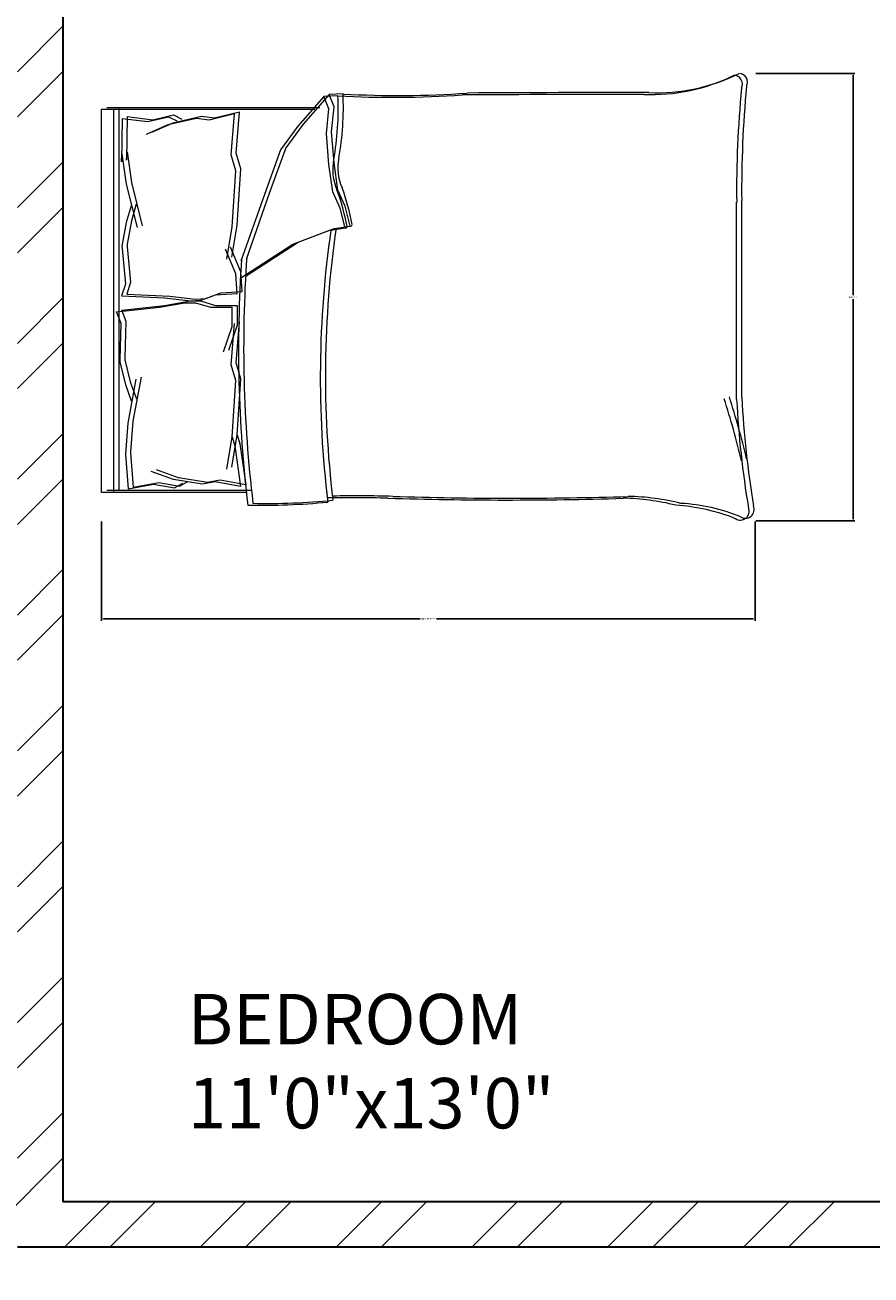
# Model space of a CAD drawing. Units: inches. Extents: x 1962 to 2771, y 1245 to 2660.
# Tile 107 of 114: x 2236 to 2319, y 2304 to 2428. Entities that reach past the tile are written whole.
import ezdxf

# ---------------------------------------------------------------- set-up
doc = ezdxf.new("R2010")
doc.units = ezdxf.units.IN
for name, color, linetype, lineweight in [('A-ANNO-DIMS', 2, 'Continuous', 18), ('A-AREA-IDEN', 7, 'Continuous', 18), ('A-FURN', 8, 'Continuous', 13), ('A-WALL', 7, 'Continuous', 35), ('A-WALL-PATT', 252, 'Continuous', 13)]:
    doc.layers.add(name, color=color, linetype=linetype, lineweight=lineweight)
doc.styles.get("Standard").update_dxf_attribs({"font": 'arial.ttf'})
doc.dimstyles.get("Standard").update_dxf_attribs({"dimtxt": 0.18, "dimasz": 0.18, "dimexe": 0.18, "dimexo": 0.0625, "dimgap": 0.09, "dimtad": 0, "dimtih": 1, "dimtoh": 1, "dimdec": 4, "dimzin": 0, "dimdsep": 46, "dimtxsty": 'Standard', "dimcen": 0.09, "dimadec": 0, "dimazin": 0, "dimtfac": 1, "dimtdec": 4, "dimtofl": 0, "dimtmove": 0, "dimatfit": 3, "dimfxl": 1, "dimtolj": 1, "dimtzin": 0, "dimarcsym": 0})

# ---------------------------------------------------------------- blocks, each defined once
blk = doc.blocks.new('BED-PLAN')
for p, q in [((22.56, 42.21), (19.98, 39.26)), ((22.56, 42.21), (19.98, 39.26)), ((23.95, 42.27), (22.56, 42.21, 3.08)), ((23.95, 42.27), (22.56, 42.21, 3.08)), ((23.06, 40.98), (22.56, 42.21)), ((23.06, 40.98), (22.56, 42.21)), ((0.51, 40.93), (21.66, 40.93)), ((0.51, 40.93), (21.66, 40.93)), ((1.73, 2.95), (1.73, 40.93)), ((1.73, 2.95), (1.73, 40.93)), ((22.05, 42.03), (19.47, 39.08)), ((22.05, 42.02), (19.47, 39.08)), ((23.44, 42.09), (22.05, 42.03, 3.08)), ((23.44, 42.09), (22.05, 42.02, 3.08)), ((22.55, 40.8), (22.05, 42.03)), ((22.55, 40.8), (22.05, 42.02)), ((22.81, 38.52), (23.06, 40.98)), ((22.81, 38.52), (23.06, 40.98)), ((0, 40.75), (21.15, 40.75)), ((0, 40.75), (21.15, 40.75)), ((0, 2.76), (0, 40.75)), ((1.22, 2.76), (1.22, 40.75)), ((1.22, 2.76), (1.22, 40.75)), ((2.03, 39.83), (1.96, 35.54)), ((2.03, 39.83), (1.96, 35.54)), ((2.03, 39.83), (4.58, 39.53)), ((2.03, 39.83), (4.58, 39.53)), ((2.54, 40.02), (2.46, 35.72)), ((2.54, 40.02), (2.46, 35.72)), ((2.54, 40.02), (5.09, 39.72)), ((2.54, 40.02), (5.09, 39.72)), ((4.58, 39.53), (6.63, 40.01)), ((4.58, 39.53), (6.63, 40.01)), ((5.09, 39.72), (7.14, 40.19)), ((5.09, 39.72), (7.14, 40.19)), ((9.4, 39.83), (6.56, 39.2)), ((9.4, 39.83), (6.56, 39.2)), ((6.63, 40.01), (7.46, 39.6)), ((6.63, 40.01), (7.46, 39.6)), ((9.91, 40.02), (7.07, 39.38)), ((9.91, 40.02), (7.07, 39.38)), ((7.14, 40.19), (7.97, 39.78)), ((7.14, 40.19), (7.97, 39.78)), ((10.68, 39.68), (9.4, 39.83)), ((10.68, 39.68), (9.4, 39.83)), ((11.19, 39.87), (9.91, 40.02)), ((11.19, 39.87), (9.91, 40.02)), ((13.17, 40.3), (10.68, 39.68)), ((13.17, 40.3), (10.68, 39.68)), ((13.68, 40.48), (11.19, 39.87)), ((13.68, 40.48), (11.19, 39.87)), ((12.85, 36.22), (13.17, 40.3)), ((12.85, 36.22), (13.17, 40.3)), ((13.36, 36.4), (13.68, 40.48)), ((13.36, 36.4), (13.68, 40.48)), ((22.3, 38.34), (22.55, 40.8)), ((22.3, 38.34), (22.55, 40.8)), ((6.56, 39.2), (4.43, 38.26)), ((6.56, 39.2), (4.43, 38.26)), ((7.07, 39.38), (4.94, 38.44)), ((7.07, 39.38), (4.94, 38.44)), ((19.47, 39.08), (17.75, 36.74)), ((19.47, 39.08), (17.75, 36.74)), ((19.98, 39.26), (18.26, 36.92)), ((19.98, 39.26), (18.26, 36.92)), ((23.06, 35.45), (22.81, 38.52)), ((23.06, 35.44), (22.81, 38.52)), ((22.55, 35.26), (22.3, 38.34)), ((22.55, 35.26), (22.3, 38.34)), ((1.96, 35.54), (2.02, 36.34)), ((1.96, 35.54), (2.02, 36.34)), ((2.02, 36.34), (2.44, 33.32)), ((2.02, 36.34), (2.44, 33.32)), ((2.46, 35.72), (2.53, 36.52)), ((2.46, 35.72), (2.53, 36.52)), ((2.53, 36.52), (2.95, 33.5)), ((2.53, 36.52), (2.95, 33.5)), ((13.3, 34.66), (12.85, 36.22)), ((13.3, 34.66), (12.85, 36.22)), ((13.8, 34.84), (13.36, 36.4)), ((13.8, 34.84), (13.36, 36.4)), ((17.75, 36.74), (16.15, 32.31)), ((17.75, 36.74), (16.15, 32.31)), ((18.26, 36.92), (16.66, 32.49)), ((18.26, 36.92), (16.66, 32.49)), ((13.46, 29.27), (13.8, 34.84)), ((13.46, 29.27), (13.8, 34.84)), ((22.92, 32.56), (22.55, 35.26)), ((22.92, 32.55), (22.55, 35.26)), ((23.42, 32.74), (23.06, 35.45)), ((23.42, 32.74), (23.06, 35.44)), ((2.95, 33.5), (4.02, 29.19)), ((2.95, 33.5), (4.02, 29.19)), ((12.95, 29.09), (13.3, 34.66)), ((12.95, 29.09), (13.3, 34.66)), ((2.44, 33.32), (3.52, 29.01)), ((2.44, 33.32), (3.52, 29.01)), ((16.15, 32.31), (13.82, 25.68)), ((16.15, 32.31), (13.82, 25.68)), ((16.66, 32.49), (14.33, 25.86)), ((16.66, 32.49), (14.33, 25.86)), ((23.65, 30.95), (22.92, 32.56)), ((23.65, 30.95), (22.92, 32.55)), ((24.16, 31.14), (23.42, 32.74)), ((24.16, 31.14), (23.42, 32.74)), ((2.92, 31.16), (2.45, 29.52)), ((2.92, 31.16), (2.45, 29.52)), ((3.43, 31.34), (2.96, 29.7)), ((3.43, 31.34), (2.96, 29.7)), ((24.65, 29.17), (24.16, 31.14)), ((24.65, 29.17), (24.16, 31.14)), ((62.99, 11.98), (62.99, 31.54)), ((62.99, 11.97), (62.99, 31.54)), ((63.5, 12.16), (63.5, 31.72)), ((63.5, 12.16), (63.5, 31.72)), ((24.15, 28.99), (23.65, 30.95)), ((24.15, 28.98), (23.65, 30.95)), ((2.45, 29.52), (2.02, 27.19)), ((2.45, 29.52), (2.02, 27.19)), ((2.96, 29.7), (2.52, 27.37)), ((2.96, 29.7), (2.52, 27.37)), ((12.42, 25.89), (12.95, 29.09)), ((12.42, 25.89), (12.95, 29.09)), ((12.93, 26.07), (13.46, 29.27)), ((12.93, 26.07), (13.46, 29.27)), ((18.98, 27.38), (22.55, 28.74)), ((18.98, 27.38), (22.55, 28.74)), ((19.49, 27.57), (23.06, 28.92)), ((19.49, 27.57), (23.06, 28.92)), ((22.55, 28.74), (24.15, 28.99)), ((22.55, 28.74), (24.15, 28.98)), ((23.06, 28.92), (24.65, 29.17)), ((23.06, 28.92), (24.65, 29.17)), ((2.52, 27.37), (2.54, 27.12)), ((2.52, 27.37), (2.54, 27.12)), ((13.82, 24.05), (18.98, 27.38)), ((13.82, 24.05), (18.98, 27.38)), ((14.33, 24.24), (19.49, 27.57)), ((14.33, 24.24), (19.49, 27.57)), ((2.02, 27.19), (2.03, 26.94)), ((2.02, 27.19), (2.03, 26.93)), ((2.03, 26.94), (2.37, 23.42)), ((2.03, 26.93), (2.37, 23.42)), ((2.54, 27.12), (2.88, 23.6)), ((2.54, 27.12), (2.88, 23.6)), ((13.31, 24.44), (12.28, 26.89)), ((13.31, 24.44), (12.28, 26.88)), ((13.81, 24.63), (12.79, 27.07)), ((13.81, 24.63), (12.79, 27.07)), ((2.88, 23.6), (2.49, 22.42)), ((2.88, 23.6), (2.49, 22.42)), ((13.43, 22.49), (13.31, 24.44)), ((13.43, 22.49), (13.31, 24.44)), ((13.94, 22.68), (13.81, 24.63)), ((13.94, 22.68), (13.81, 24.63)), ((2.37, 23.42), (1.98, 22.24)), ((2.37, 23.42), (1.98, 22.24)), ((2.49, 22.42), (6.76, 22.23)), ((2.49, 22.42), (6.76, 22.23)), ((9.84, 21.81), (11.3, 22.36)), ((9.84, 21.81), (11.3, 22.36)), ((10.35, 21.99), (11.81, 22.54)), ((10.35, 21.99), (11.81, 22.54)), ((11.3, 22.36), (13.43, 22.49)), ((11.3, 22.36), (13.43, 22.49)), ((11.81, 22.54), (13.94, 22.68)), ((11.81, 22.54), (13.94, 22.68)), ((1.49, 20.65), (5.74, 21.11)), ((1.49, 20.65), (5.74, 21.11)), ((1.98, 22.24), (6.25, 22.05)), ((1.98, 22.24), (6.25, 22.05)), ((1.99, 20.84), (6.25, 21.3)), ((1.99, 20.84), (6.25, 21.3)), ((5.74, 21.11), (8.27, 21.57)), ((5.74, 21.11), (8.27, 21.57)), ((6.25, 22.05), (8.81, 21.75)), ((6.25, 22.05), (8.81, 21.75)), ((6.25, 21.3), (8.78, 21.76)), ((6.25, 21.3), (8.78, 21.76)), ((6.76, 22.23), (9.31, 21.93)), ((6.76, 22.23), (9.31, 21.93)), ((8.27, 21.57), (9.3, 21.57)), ((8.27, 21.57), (9.3, 21.57)), ((8.78, 21.76), (9.81, 21.76)), ((8.78, 21.76), (9.81, 21.76)), ((8.81, 21.75), (9.84, 21.81)), ((8.81, 21.75), (9.84, 21.81)), ((9.3, 21.57), (10.8, 21.11)), ((9.3, 21.57), (10.8, 21.11)), ((9.31, 21.93), (10.35, 21.99)), ((9.31, 21.93), (10.35, 21.99)), ((9.81, 21.76), (11.3, 21.3)), ((9.81, 21.76), (11.3, 21.3)), ((10.8, 21.11), (12.93, 21.11)), ((10.8, 21.11), (12.93, 21.11)), ((11.3, 21.3), (13.44, 21.3)), ((11.3, 21.3), (13.44, 21.3)), ((12.93, 21.11), (12.93, 19.16)), ((12.93, 21.11), (12.93, 19.16)), ((13.44, 21.3), (13.44, 19.34)), ((13.44, 21.3), (13.44, 19.34)), ((1.95, 19.51), (1.49, 20.65)), ((1.95, 19.51), (1.49, 20.65)), ((2.45, 19.69), (1.99, 20.84)), ((2.45, 19.69), (1.99, 20.84)), ((1.83, 15.97), (1.95, 19.51)), ((1.83, 15.97), (1.95, 19.51)), ((2.34, 16.15), (2.45, 19.69)), ((2.34, 16.15), (2.45, 19.69)), ((12.93, 19.16), (12.06, 16.66)), ((12.93, 19.16), (12.06, 16.66)), ((13.44, 19.34), (12.57, 16.84)), ((13.44, 19.34), (12.57, 16.84)), ((12.85, 15.41), (13.17, 19.49)), ((12.85, 15.41), (13.17, 19.49)), ((13.36, 15.59), (13.68, 19.67)), ((13.36, 15.59), (13.68, 19.67)), ((2.34, 15.9), (2.34, 16.15)), ((2.34, 15.9), (2.34, 16.15)), ((1.83, 15.72), (1.83, 15.97)), ((1.83, 15.72), (1.83, 15.97)), ((2.41, 13.42), (1.83, 15.72)), ((2.41, 13.42), (1.83, 15.72)), ((2.91, 13.6), (2.34, 15.9)), ((2.91, 13.6), (2.34, 15.9)), ((13.3, 13.85), (12.85, 15.41)), ((13.3, 13.85), (12.85, 15.41)), ((13.8, 14.03), (13.36, 15.59)), ((13.8, 14.03), (13.36, 15.59)), ((2.64, 9.63), (3.44, 13.99)), ((2.64, 9.63), (3.44, 13.99)), ((3.14, 9.81), (3.95, 14.17)), ((3.14, 9.81), (3.95, 14.17)), ((12.95, 8.28), (13.3, 13.85)), ((12.95, 8.28), (13.3, 13.85)), ((13.46, 8.46), (13.8, 14.03)), ((13.46, 8.46), (13.8, 14.03)), ((2.98, 11.81), (2.41, 13.42)), ((2.98, 11.81), (2.41, 13.42)), ((3.49, 11.99), (2.91, 13.6)), ((3.49, 11.99), (2.91, 13.6)), ((2.41, 6.59), (2.64, 9.63)), ((2.41, 6.59), (2.64, 9.63)), ((2.91, 6.77), (3.14, 9.81)), ((2.91, 6.77), (3.14, 9.81)), ((12.42, 5.07), (12.95, 8.28)), ((12.42, 5.07), (12.95, 8.28)), ((12.93, 5.26), (13.46, 8.46)), ((12.93, 5.26), (13.46, 8.46)), ((12.95, 8.28), (13.21, 7.38)), ((12.95, 8.28), (13.21, 7.38)), ((13.46, 8.46), (13.72, 7.56)), ((13.46, 8.46), (13.72, 7.56)), ((13.72, 7.56), (14.29, 3.51)), ((13.72, 7.56), (14.29, 3.51)), ((2.39, 6.5), (2.41, 6.59)), ((2.39, 6.5), (2.41, 6.59)), ((2.65, 3.1), (2.39, 6.5)), ((2.65, 3.1), (2.39, 6.5)), ((2.9, 6.68), (2.91, 6.77)), ((2.9, 6.68), (2.91, 6.77)), ((3.16, 3.28), (2.9, 6.68)), ((3.16, 3.28), (2.9, 6.68)), ((13.21, 7.38), (13.78, 3.33)), ((13.21, 7.38), (13.78, 3.33)), ((7.63, 4.2), (5.44, 5)), ((7.63, 4.2), (5.44, 5)), ((3.14, 3.28), (5.67, 3.74)), ((3.14, 3.28), (5.67, 3.74)), ((7.12, 4.02), (4.93, 4.82)), ((7.12, 4.02), (4.93, 4.82)), ((5.67, 3.74), (7.74, 3.39)), ((5.67, 3.74), (7.74, 3.39)), ((9.99, 3.56), (7.12, 4.02)), ((9.99, 3.56), (7.12, 4.02)), ((10.5, 3.74), (7.63, 4.2)), ((10.5, 3.74), (7.63, 4.2)), ((7.74, 3.39), (8.55, 3.85)), ((7.74, 3.39), (8.55, 3.85)), ((11.26, 3.79), (9.99, 3.56)), ((11.26, 3.79), (9.99, 3.56)), ((11.76, 3.97), (10.5, 3.74)), ((11.76, 3.97), (10.5, 3.74)), ((13.78, 3.33), (11.26, 3.79)), ((13.78, 3.33), (11.26, 3.79)), ((14.29, 3.51), (11.76, 3.97)), ((14.29, 3.51), (11.76, 3.97)), ((14.4, 2.76), (0, 2.76)), ((14.4, 2.76), (0, 2.76)), ((14.9, 2.95), (0.51, 2.95)), ((14.9, 2.95), (0.51, 2.95)), ((2.64, 3.1), (5.16, 3.56)), ((2.64, 3.1), (5.16, 3.56)), ((5.16, 3.56), (7.23, 3.21)), ((5.16, 3.56), (7.23, 3.21)), ((7.23, 3.21), (8.04, 3.67)), ((7.23, 3.21), (8.04, 3.67))]:
    blk.add_line(p, q)
for centre, radius, start, end in [((54.58, 60.54), 18.33, 267.4714, 296.4681), ((54.58, 60.54), 18.33, 267.4714, 296.4681), ((55.09, 60.72), 18.33, 267.4714, 296.4681), ((55.09, 60.72), 18.33, 267.4714, 296.4681), ((62.69, 43.25), 0.876, 332.6588, 86.02), ((62.69, 43.25), 0.876, 332.6588, 86.02), ((63.2, 43.43), 0.876, 332.6588, 86.02), ((63.2, 43.43), 0.876, 332.6588, 86.02), ((28.87, 144.88), 102.94, 266.9791, 273.8365), ((28.87, 144.88), 102.94, 266.9791, 273.8365), ((-4.78, 40.98), 28.76, 349.8763, 2.5657), ((-4.78, 40.98), 28.76, 349.8763, 2.5657), ((29.37, 145.06), 102.94, 266.9791, 273.8365), ((29.37, 145.06), 102.94, 266.9791, 273.8365), ((53.91, -3583.94), 3626.16, 90.00217, 90.28689), ((53.91, -3583.94), 3626.16, 90.00217, 90.28689), ((54.42, -3583.75), 3626.16, 90.00217, 90.28689), ((54.42, -3583.75), 3626.16, 90.00217, 90.28689), ((168.74, 32.71), 105.75, 174.4998, 180.6351), ((168.74, 32.71), 105.75, 174.4998, 180.6351), ((169.24, 32.89), 105.75, 174.4998, 180.6351), ((169.24, 32.89), 105.75, 174.4998, 180.6351), ((-5.29, 40.8), 28.76, 349.8763, 2.5657), ((-5.29, 40.8), 28.76, 349.8763, 2.5657), ((27.87, 34.77), 4.95, 168.6608, 203.7384), ((27.87, 34.77), 4.95, 168.6608, 203.7384), ((28.38, 34.95), 4.95, 168.6608, 203.7384), ((28.38, 34.95), 4.95, 168.6608, 203.7384), ((1.18, 24.77), 23.57, 10.6617, 19.8806), ((1.18, 24.76), 23.57, 10.6617, 19.8806), ((1.69, 24.95), 23.57, 10.6617, 19.8806), ((1.69, 24.95), 23.57, 10.6617, 19.8806), ((124.25, 14.12), 102.56, 171.7845, 186.9006), ((124.25, 14.11), 102.56, 171.7845, 186.9006), ((124.76, 14.3), 102.56, 171.7845, 186.9006), ((124.76, 14.3), 102.56, 171.7845, 186.9006), ((24.2, 29.12), 0.147, 250.2464, 1.1377), ((24.2, 29.12), 0.147, 250.2464, 1.1377), ((24.7, 29.3), 0.147, 250.2464, 1.1377), ((24.7, 29.3), 0.147, 250.2464, 1.1377), ((145.22, 17.16), 131.13, 176.0865, 186.7821), ((145.22, 17.16), 131.13, 176.0865, 186.7821), ((144.71, 16.98), 131.13, 176.0865, 186.7821), ((144.71, 16.98), 131.13, 176.0865, 186.7821), ((-18.85, -13.69), 84.62, 13.3832, 17.7053), ((-18.85, -13.69), 84.62, 13.3832, 17.7053), ((-18.34, -13.51), 84.62, 13.3832, 17.7053), ((-18.34, -13.51), 84.62, 13.3832, 17.7053), ((159.64, 17.03), 96.78, 182.9958, 189.4091), ((159.64, 17.03), 96.78, 182.9958, 189.4091), ((160.15, 17.21), 96.78, 182.9958, 189.4091), ((160.15, 17.21), 96.78, 182.9958, 189.4091), ((15.97, 67.7), 66.22, 268.7218, 275.604), ((15.97, 67.7), 66.22, 268.7218, 275.604), ((16.48, 67.88), 66.22, 268.7218, 275.604), ((16.48, 67.88), 66.22, 268.7218, 275.604), ((24.78, -132.99), 135.22, 88.4762, 91.0082), ((24.78, -132.99), 135.22, 88.4762, 91.0082), ((25.29, -132.81), 135.22, 88.4762, 91.0082), ((25.29, -132.81), 135.22, 88.4762, 91.0082), ((40.23, 385.38), 383.38, 268.2277, 271.7185), ((40.23, 385.38), 383.38, 268.2277, 271.7185), ((40.74, 385.56), 383.38, 268.2277, 271.7185), ((40.74, 385.56), 383.38, 268.2277, 271.7185), ((51.28, -21.38), 23.56, 76.0648, 88.9113), ((51.28, -21.38), 23.56, 76.0648, 88.9113), ((51.79, -21.2), 23.56, 76.0648, 88.9113), ((51.79, -21.2), 23.56, 76.0648, 88.9113), ((55.86, -17.22), 18.73, 67.9751, 86.652), ((55.86, -17.22), 18.73, 67.9751, 86.652), ((56.37, -17.03), 18.73, 67.9751, 86.652), ((56.37, -17.03), 18.73, 67.9751, 86.652), ((63.87, 1.05), 0.866, 236.1736, 23.4781), ((63.87, 1.05), 0.866, 236.1736, 23.4781), ((63.37, 0.87), 0.866, 236.1736, 23.4781), ((63.37, 0.87), 0.866, 236.1736, 23.4781)]:
    blk.add_arc(centre, radius, start, end)
blk = doc.blocks.new('*D14')
at = {"layer": 'A-ANNO-DIMS', "color": 0, "lineweight": -2, "transparency": 16777216}
for p, q in [((2243.15, 2378.79), (2243.15, 2368.94)), ((2307.97, 2378.79), (2307.97, 2368.94)), ((2243.33, 2369.12), (2274.74, 2369.12)), ((2307.79, 2369.12), (2276.38, 2369.12))]:
    blk.add_line(p, q, dxfattribs=at)
at = {"layer": 'A-ANNO-DIMS', "color": 0, "transparency": 16777216}
for points in [[(2243.33, 2369.15), (2243.33, 2369.09), (2243.15, 2369.12)], [(2307.79, 2369.15), (2307.79, 2369.09), (2307.97, 2369.12)]]:
    blk.add_solid(points, dxfattribs=at)
at = {"layer": 'Defpoints', "color": 0, "transparency": 16777216}
for p in [(2243.15, 2378.85), (2307.97, 2378.85), (2307.97, 2369.12)]:
    blk.add_point(p, dxfattribs=at)
at = {"layer": 'A-ANNO-DIMS', "color": 0, "transparency": 16777216, "insert": (2275.56, 2369.12), "char_height": 0.18, "attachment_point": 5}
blk.add_mtext('\\A1;BED 65 TYP.', dxfattribs=at)
blk = doc.blocks.new('*D15')
at = {"layer": 'A-ANNO-DIMS', "color": 0, "lineweight": -2, "transparency": 16777216}
for p, q in [((2308.03, 2423.22), (2317.87, 2423.22)), ((2317.69, 2423.04), (2317.69, 2401.22)), ((2317.69, 2379.03), (2317.69, 2400.85)), ((2308.03, 2378.85), (2317.87, 2378.85))]:
    blk.add_line(p, q, dxfattribs=at)
at = {"layer": 'A-ANNO-DIMS', "color": 0, "transparency": 16777216}
for points in [[(2317.66, 2423.04), (2317.72, 2423.04), (2317.69, 2423.22)], [(2317.66, 2379.03), (2317.72, 2379.03), (2317.69, 2378.85)]]:
    blk.add_solid(points, dxfattribs=at)
at = {"layer": 'Defpoints', "color": 0, "transparency": 16777216}
for p in [(2307.97, 2423.22), (2317.69, 2423.22), (2307.97, 2378.85)]:
    blk.add_point(p, dxfattribs=at)
at = {"layer": 'A-ANNO-DIMS', "color": 0, "transparency": 16777216, "insert": (2317.69, 2401.03), "char_height": 0.18, "attachment_point": 5}
blk.add_mtext('\\A1;44 TYP.', dxfattribs=at)
blk = doc.blocks.new('*D40')
at = {"layer": 'A-ANNO-DIMS', "color": 0, "lineweight": -2, "transparency": 16777216}
for p, q in [((2072.02, 2033.91), (2072.02, 2583.47)), ((2660.81, 2524.41), (2660.81, 2583.47)), ((2072.2, 2583.29), (2366.02, 2583.29)), ((2660.63, 2583.29), (2366.81, 2583.29))]:
    blk.add_line(p, q, dxfattribs=at)
at = {"layer": 'A-ANNO-DIMS', "color": 0, "transparency": 16777216}
for points in [[(2072.2, 2583.32), (2072.2, 2583.26), (2072.02, 2583.29)], [(2660.63, 2583.32), (2660.63, 2583.26), (2660.81, 2583.29)]]:
    blk.add_solid(points, dxfattribs=at)
at = {"layer": 'Defpoints', "color": 0, "transparency": 16777216}
for p in [(2660.81, 2583.29), (2660.81, 2524.34), (2072.02, 2033.84)]:
    blk.add_point(p, dxfattribs=at)
at = {"layer": 'A-ANNO-DIMS', "color": 0, "transparency": 16777216, "insert": (2366.41, 2583.29), "char_height": 0.18, "attachment_point": 5}
blk.add_mtext('\\A1;588.8', dxfattribs=at)

msp = doc.modelspace()

# ---------------------------------------------------------------- hatches: boundary and pattern name
at = {"layer": 'A-WALL-PATT'}
h = msp.add_hatch(dxfattribs=at)
h.set_pattern_fill('ANSI32', color=256)
h.paths.add_polyline_path([(2090.8074, 2467.3437), (2141.6481, 2467.3437), (2141.6481, 2469.5937), (2141.6481, 2471.8437), (2086.3074, 2471.8437), (2086.3074, 2422.5333), (2090.8074, 2422.5333)])
h.paths.add_polyline_path([(2282.7664, 2471.8437), (2204.8982, 2471.8437), (2204.8982, 2467.3437), (2234.8074, 2467.3437), (2234.8074, 2311.3437), (2228.7492, 2311.3437), (2228.7492, 2306.8437), (2234.8074, 2306.8437), (2331.9227, 2306.8437), (2331.9227, 2309.0937), (2331.9227, 2311.3437), (2239.3074, 2311.3437), (2239.3074, 2467.3437), (2282.7664, 2467.3437), (2282.7664, 2469.5937)])
h.paths.add_polyline_path([(2471.4531, 2519.8437), (2552.011, 2519.8437), (2564.3996, 2519.8437), (2564.3996, 2511.1389), (2568.8996, 2511.1389), (2568.8996, 2524.3437), (2466.9531, 2524.3437), (2466.9531, 2471.8437), (2450.0749, 2471.8437), (2446.4672, 2471.8437), (2446.4672, 2467.3437), (2450.0749, 2467.3437), (2475.9988, 2467.3437), (2475.9988, 2469.5937), (2475.9988, 2471.8437), (2471.4531, 2471.8437)])
h.paths.add_polyline_path([(2575.2231, 2469.5937), (2575.2231, 2471.8437), (2568.8996, 2471.8437), (2568.8996, 2487.1389), (2564.3996, 2487.1389), (2564.3996, 2471.8437), (2556.511, 2471.8437), (2499.2904, 2471.8437), (2499.2904, 2467.3437), (2507.8074, 2467.3437), (2507.8074, 2311.3437), (2414.863, 2311.3437), (2414.863, 2306.8437), (2512.3074, 2306.8437), (2517.0114, 2306.8437), (2517.0114, 2309.0937), (2517.0114, 2311.3437), (2512.3074, 2311.3437), (2512.3074, 2467.3437), (2575.2231, 2467.3437)])
h.paths.add_polyline_path([(2660.8074, 2471.8437), (2600.9602, 2471.8437), (2600.9602, 2467.3437), (2656.3074, 2467.3437), (2656.3074, 2432.5704), (2660.8074, 2432.5704)])
h.paths.add_polyline_path([(2660.8074, 2372.5704), (2656.3074, 2372.5704), (2656.3074, 2311.3437), (2600.276, 2311.3437), (2600.276, 2309.0937), (2600.276, 2306.8437), (2656.3074, 2306.8437), (2656.3074, 2296.2593), (2660.8074, 2296.2593)])
h.paths.add_polyline_path([(2572.3074, 2306.8437), (2577.1385, 2306.8437), (2577.1385, 2311.3437), (2551.082, 2311.3437), (2551.082, 2306.8437), (2567.8074, 2306.8437), (2567.8074, 2258.8437), (2540.0574, 2258.8437), (2540.0574, 2256.5937), (2540.0574, 2254.3437), (2567.8074, 2254.3437), (2656.3074, 2254.3437), (2656.3074, 2236.9085), (2660.8074, 2236.9085), (2660.8074, 2272.2593), (2656.3074, 2272.2593), (2656.3074, 2258.8437), (2572.3074, 2258.8437)])
h.paths.add_polyline_path([(2512.3074, 2254.3437), (2518.8716, 2254.3437), (2518.8716, 2256.5937), (2518.8716, 2258.8437), (2507.8074, 2258.8437), (2507.8074, 2177.8437), (2567.8074, 2177.8437), (2567.8074, 2172.9628), (2572.3074, 2172.9628), (2572.3074, 2177.8437), (2656.3074, 2177.8437), (2656.3074, 2166.4846), (2660.8074, 2166.4846), (2660.8074, 2200.9085), (2656.3074, 2200.9085), (2656.3074, 2182.3437), (2512.3074, 2182.3437)])
h.paths.add_polyline_path([(2656.3074, 2129.8437), (2572.3074, 2129.8437), (2572.3074, 2150.3044), (2570.0574, 2150.3044), (2567.8074, 2150.3044), (2567.8074, 2129.8437), (2507.8074, 2129.8437), (2507.8074, 2116.3027), (2510.0574, 2116.3027), (2512.3074, 2116.3027), (2512.3074, 2125.3437), (2567.8074, 2125.3437), (2572.3074, 2125.3437), (2656.3074, 2125.3437)])
h.paths.add_polyline_path([(2090.8074, 2362.5333), (2086.3074, 2362.5333), (2086.3074, 2298.6242), (2090.8074, 2298.6242), (2090.8074, 2306.8437), (2174.8074, 2306.8437), (2174.8074, 2286.4178), (2179.3074, 2286.4178), (2179.3074, 2306.8437), (2192.8641, 2306.8437), (2192.8641, 2309.0937), (2192.8641, 2311.3437), (2090.8074, 2311.3437)])
h.paths.add_polyline_path([(2209.156, 2258.8437), (2179.3074, 2258.8437), (2179.3074, 2263.2236), (2177.0574, 2263.2236), (2174.8074, 2263.2236), (2174.8074, 2258.8437), (2090.8074, 2258.8437), (2090.8074, 2274.6242), (2086.3074, 2274.6242), (2086.3074, 2238.2967), (2088.5574, 2238.2967), (2090.8074, 2238.2967), (2090.8074, 2254.3437), (2209.156, 2254.3437)])
h.paths.add_polyline_path([(2090.8074, 2177.8437), (2234.8074, 2177.8437), (2234.8074, 2173.1428), (2239.3074, 2173.1428), (2239.3074, 2258.8437), (2230.8442, 2258.8437), (2230.8442, 2256.5937), (2230.8442, 2254.3437), (2234.8074, 2254.3437), (2234.8074, 2182.3437), (2090.8074, 2182.3437), (2090.8074, 2202.2967), (2086.3074, 2202.2967), (2086.3074, 2140.0389), (2090.8074, 2140.0389)])
h.paths.add_polyline_path([(2090.8074, 2080.0389), (2086.3074, 2080.0389), (2086.3074, 2033.8437), (2090.8074, 2033.8437)], flags=17)
h.paths.add_polyline_path([(2244.9405, 2033.8437), (2239.3074, 2033.8437), (2239.3074, 2142.0665), (2237.2592, 2142.0665), (2234.8074, 2142.0665), (2234.8074, 2033.8437), (2090.8074, 2033.8437), (2076.5204, 2033.8437), (2072.0204, 2033.8437), (2072.0204, 2000.4493), (2076.5204, 2000.4493), (2076.5204, 2029.3437), (2090.8074, 2029.3437), (2244.9405, 2029.3437), (2244.9405, 2031.5937)])
h.paths.add_polyline_path([(2234.8074, 1933.3437), (2076.5204, 1933.3437), (2076.5204, 1952.4493), (2074.2704, 1952.4493), (2072.0204, 1952.4493), (2072.0204, 1933.3437), (2072.0204, 1928.8437), (2234.8074, 1928.8437)])
h.paths.add_polyline_path([(2090.8074, 1928.8437), (2086.3074, 1928.8437), (2086.3074, 1906.5013), (2090.8074, 1906.5013)])
h.paths.add_polyline_path([(2090.8074, 1846.5013), (2086.3074, 1846.5013), (2086.3074, 1769.9917), (2088.5574, 1769.9917), (2090.8074, 1769.9917), (2090.8074, 1780.3437), (2234.8074, 1780.3437), (2234.8074, 1708.3437), (2230.3764, 1708.3437), (2230.3764, 1703.8437), (2239.3074, 1703.8437), (2239.3074, 1792.6669), (2237.0574, 1792.6669), (2234.8074, 1792.6669), (2234.8074, 1784.8437), (2090.8074, 1784.8437)])
h.paths.add_polyline_path([(2239.3074, 1928.8437), (2244.9405, 1928.8437), (2244.9405, 1931.0937), (2244.9405, 1933.3437), (2234.8074, 1933.3437), (2234.8074, 1928.8437), (2234.8074, 1825.5949), (2239.3074, 1825.5949)])
h.paths.add_polyline_path([(2148.0425, 1649.0937), (2148.0425, 1651.3437), (2090.8074, 1651.3437), (2090.8074, 1646.8437), (2148.0425, 1646.8437)], flags=0)
h.paths.add_polyline_path([(2207.5601, 1708.3437), (2090.8074, 1708.3437), (2090.8074, 1703.8437), (2174.8074, 1703.8437), (2174.8074, 1651.3437), (2170.4457, 1651.3437), (2170.4457, 1646.8437), (2195.9924, 1646.8437), (2195.9924, 1649.0937), (2195.9924, 1651.3437), (2179.3074, 1651.3437), (2179.3074, 1703.8437), (2207.5601, 1703.8437), (2207.5601, 1706.0937)])
h.paths.add_polyline_path([(2090.8074, 1733.9917), (2086.3074, 1733.9917), (2086.3074, 1696.1032), (2088.5574, 1696.1032), (2090.8074, 1696.1032)])
h.paths.add_polyline_path([(2090.8074, 1672.1032), (2086.3074, 1672.1032), (2086.3074, 1600.3335), (2090.8074, 1600.3335)])
h.paths.add_polyline_path([(2090.8074, 1540.3335), (2086.3074, 1540.3335), (2086.3074, 1486.3437), (2139.6766, 1486.3437), (2139.6766, 1490.8437), (2090.8074, 1490.8437)])
h.paths.add_polyline_path([(2302.3876, 1490.8437), (2239.3074, 1490.8437), (2239.3074, 1646.8437), (2335.9994, 1646.8437), (2335.9994, 1651.3437), (2229.884, 1651.3437), (2229.884, 1646.8437), (2234.8074, 1646.8437), (2234.8074, 1490.8437), (2202.7103, 1490.8437), (2202.7103, 1488.5937), (2202.7103, 1486.3437), (2275.0699, 1486.3437), (2275.0699, 1475.772), (2279.5699, 1475.772), (2279.5699, 1486.3437), (2302.3876, 1486.3437)])
h.paths.add_polyline_path([(2279.5699, 1451.772), (2275.0699, 1451.772), (2275.0699, 1438.3437), (2174.8074, 1438.3437), (2174.8074, 1486.3437), (2179.7922, 1486.3437), (2179.7922, 1490.8437), (2163.3585, 1490.8437), (2163.3585, 1488.5937), (2163.3585, 1486.3437), (2170.3074, 1486.3437), (2170.3074, 1433.8437), (2279.5699, 1433.8437)])
h.paths.add_polyline_path([(2427.2363, 1490.8437), (2375.8074, 1490.8437), (2375.8074, 1646.8437), (2381.6401, 1646.8437), (2381.6401, 1651.3437), (2365.887, 1651.3437), (2365.887, 1649.0937), (2365.887, 1646.8437), (2371.3074, 1646.8437), (2371.3074, 1490.8437), (2327.5627, 1490.8437), (2327.5627, 1488.5937), (2327.5627, 1486.3437), (2371.3074, 1486.3437), (2371.3074, 1433.8437), (2375.8074, 1433.8437), (2375.8074, 1486.3437), (2427.2363, 1486.3437)])
h.paths.add_polyline_path([(2512.3074, 1646.8437), (2519.4351, 1646.8437), (2519.4351, 1649.0937), (2519.4351, 1651.3437), (2507.8074, 1651.3437), (2416.0063, 1651.3437), (2416.0063, 1649.0937), (2416.0063, 1646.8437), (2507.8074, 1646.8437), (2507.8074, 1490.8437), (2497.0532, 1490.8437), (2497.0532, 1488.5937), (2497.0532, 1486.3437), (2574.9344, 1486.3437), (2574.9344, 1476.0181), (2579.4344, 1476.0181), (2579.4344, 1486.3437), (2584.4872, 1486.3437), (2584.3074, 1490.8437), (2512.3074, 1490.8437)])
h.paths.add_polyline_path([(2470.5091, 1486.3437), (2473.9767, 1486.3437), (2473.9767, 1490.8437), (2449.6605, 1490.8437), (2449.6605, 1488.5937), (2449.6605, 1486.3437), (2466.0091, 1486.3437), (2466.0091, 1433.8437), (2470.5091, 1433.8437), (2579.4344, 1433.8437), (2579.4344, 1452.0181), (2574.9344, 1452.0181), (2574.9344, 1438.3437), (2554.5091, 1438.3437), (2470.5091, 1438.3437)])
h.paths.add_polyline_path([(2656.3074, 1490.8437), (2611.86, 1490.8437), (2611.86, 1486.3437), (2656.3074, 1486.3437)])
h.paths.add_polyline_path([(2660.8074, 1532.7007), (2658.5574, 1532.7007), (2656.3074, 1532.7007), (2656.3074, 1486.3437), (2660.8074, 1486.3437)])
h.paths.add_polyline_path([(2660.8074, 1664.9663), (2656.3074, 1664.9663), (2656.3074, 1651.3437), (2602.2313, 1651.3437), (2602.2313, 1646.8437), (2656.3074, 1646.8437), (2656.3074, 1592.7007), (2660.8074, 1592.7007)])
h.paths.add_polyline_path([(2660.8074, 1724.5221), (2656.3074, 1724.5221), (2656.3074, 1703.8437), (2542.4725, 1703.8437), (2542.4725, 1699.3437), (2567.8074, 1699.3437), (2567.8074, 1651.3437), (2552.7766, 1651.3437), (2552.7766, 1649.0937), (2552.7766, 1646.8437), (2577.2878, 1646.8437), (2577.2878, 1649.0937), (2577.2878, 1651.3437), (2572.3074, 1651.3437), (2572.3074, 1699.3437), (2656.3074, 1699.3437), (2656.3074, 1688.9663), (2660.8074, 1688.9663)])
h.paths.add_polyline_path([(2660.8074, 1880.6524), (2656.3074, 1880.6524), (2656.3074, 1832.8437), (2512.3074, 1832.8437), (2512.3074, 1837.8959), (2507.8074, 1837.8959), (2507.8074, 1828.3437), (2567.8074, 1828.3437), (2567.8074, 1804.3437), (2572.3074, 1804.3437), (2572.3074, 1828.3437), (2656.3074, 1828.3437), (2656.3074, 1818.6778), (2660.8074, 1818.6778)])
h.paths.add_polyline_path([(2660.8074, 1794.6778), (2656.3074, 1794.6778), (2656.3074, 1780.3437), (2572.3074, 1780.3437), (2572.3074, 1783.0303), (2570.0574, 1783.0303), (2567.8074, 1783.0303), (2567.8074, 1780.3437), (2507.8074, 1780.3437), (2507.8074, 1699.3437), (2517.8858, 1699.3437), (2517.8858, 1701.5937), (2517.8858, 1703.8437), (2512.3074, 1703.8437), (2512.3074, 1775.8437), (2656.3074, 1775.8437), (2656.3074, 1760.5221), (2660.8074, 1760.5221)])
h.paths.add_polyline_path([(2660.8074, 1981.3437), (2660.8074, 2020.2808), (2658.5574, 2020.2808), (2656.3074, 2020.2808), (2656.3074, 1981.3437), (2512.3074, 1981.3437), (2512.3074, 2086.6996), (2507.8074, 2086.6996), (2507.8074, 1981.3437), (2375.8074, 1981.3437), (2375.8074, 1986.8505), (2373.5574, 1986.8505), (2371.3074, 1986.8505), (2371.3074, 1973.2607), (2375.8074, 1973.2607), (2375.8074, 1976.8437), (2507.8074, 1976.8437), (2507.8074, 1865.4281), (2510.0574, 1865.4281), (2512.3074, 1865.4281), (2512.3074, 1976.8437), (2660.8074, 1976.8437)])
h.paths.add_polyline_path([(2375.8074, 1940.297), (2373.5574, 1940.297), (2371.3074, 1940.297), (2371.3074, 1933.3437), (2278.4434, 1933.3437), (2278.4434, 1928.8437), (2371.3074, 1928.8437), (2371.3074, 1651.3437), (2375.8074, 1651.3437)])
h.paths.add_polyline_path([(2660.8074, 1976.8437), (2656.3074, 1976.8437), (2656.3074, 1940.6524), (2660.8074, 1940.6524)], flags=17)
h.paths.add_polyline_path([(2660.8074, 2142.4846), (2656.3074, 2142.4846), (2656.3074, 2080.2808), (2660.8074, 2080.2808)])
h.paths.add_polyline_path([(2381.4189, 2311.3437), (2375.8074, 2311.3437), (2375.8074, 2467.3437), (2424.7242, 2467.3437), (2424.7242, 2469.5937), (2424.7242, 2471.8437), (2375.8074, 2471.8437), (2375.8074, 2524.3437), (2371.3074, 2524.3437), (2371.3074, 2471.8437), (2307.2097, 2471.8437), (2307.2097, 2467.3437), (2371.3074, 2467.3437), (2371.3074, 2311.3437), (2366.8901, 2311.3437), (2366.8901, 2306.8437), (2371.3074, 2306.8437), (2371.3074, 2033.8437), (2279.6589, 2033.8437), (2279.6589, 2029.3437), (2371.3074, 2029.3437), (2371.3074, 2014.2598), (2375.8074, 2014.2598), (2375.8074, 2306.8437), (2381.4189, 2306.8437)])
h.paths.add_polyline_path([(2263.3074, 2524.3437), (2170.3074, 2524.3437), (2170.3074, 2519.8437), (2170.3074, 2471.8437), (2165.0312, 2471.8437), (2165.0312, 2467.3437), (2179.6721, 2467.3437), (2179.6721, 2469.5161), (2179.6721, 2471.8437), (2174.8074, 2471.8437), (2174.8074, 2519.8437), (2258.8074, 2519.8437), (2258.8074, 2511.6436), (2263.3074, 2511.6436)])
h.paths.add_polyline_path([(2245.0232, 1361.4123), (2492.9468, 1361.4123), (2492.9468, 1398.505), (2245.0232, 1398.505)], flags=9)
h.paths.add_polyline_path([(2388.1434, 2086.6936), (2425.0704, 2086.6936), (2425.0704, 2105.3509), (2388.1434, 2105.3509)], flags=9)
h.paths.add_polyline_path([(2404.922, 2242.6744), (2445.7337, 2242.6744), (2445.7337, 2261.3318), (2404.922, 2261.3318)], flags=9)
h.paths.add_polyline_path([(2269.4107, 2156.7935), (2306.3378, 2156.7935), (2306.3378, 2175.4508), (2269.4107, 2175.4508)], flags=9)
h.paths.add_polyline_path([(2269.3277, 2233.4343), (2306.2547, 2233.4343), (2306.2547, 2252.0917), (2269.3277, 2252.0917)], flags=9)
h.paths.add_polyline_path([(2431.6052, 2320.6922), (2470.4456, 2320.6922), (2470.4456, 2339.3495), (2431.6052, 2339.3495)], flags=25)
h.paths.add_polyline_path([(2249.6902, 2315.7608), (2288.5306, 2315.7608), (2288.5306, 2334.4182), (2249.6902, 2334.4182)], flags=25)
h.paths.add_polyline_path([(2096.9301, 2314.3181), (2135.7704, 2314.3181), (2135.7704, 2332.9755), (2096.9301, 2332.9755)], flags=25)
h.paths.add_polyline_path([(2134.3475, 2285.7089), (2161.4655, 2285.7089), (2161.4655, 2304.3662), (2134.3475, 2304.3662)], flags=9)
h.paths.add_polyline_path([(2126.5155, 2209.4076), (2159.9227, 2209.4076), (2159.9227, 2228.065), (2126.5155, 2228.065)], flags=25)
h.paths.add_polyline_path([(2110.5753, 2141.5299), (2149.4157, 2141.5299), (2149.4157, 2160.1872), (2110.5753, 2160.1872)], flags=25)
h.paths.add_polyline_path([(2249.8618, 1968.3317), (2286.3966, 1968.3317), (2286.3966, 1986.989), (2249.8618, 1986.989)], flags=9)
h.paths.add_polyline_path([(2395.9507, 1777.0051), (2436.7624, 1777.0051), (2436.7624, 1795.6625), (2395.9507, 1795.6625)], flags=9)
h.paths.add_polyline_path([(2398.5259, 1888.5651), (2435.0062, 1888.5651), (2435.0062, 1907.2224), (2398.5259, 1907.2224)], flags=25)
h.paths.add_polyline_path([(2259.3506, 1728.3559), (2296.2776, 1728.3559), (2296.2776, 1747.0132), (2259.3506, 1747.0132)], flags=9)
h.paths.add_polyline_path([(2271.3698, 1845.268), (2308.2968, 1845.268), (2308.2968, 1863.9253), (2271.3698, 1863.9253)], flags=9)
h.paths.add_polyline_path([(2120.9355, 1786.3027), (2159.7759, 1786.3027), (2159.7759, 1804.9601), (2120.9355, 1804.9601)], flags=25)
h.paths.add_polyline_path([(2121.3164, 1732.1043), (2154.7236, 1732.1043), (2154.7236, 1750.7616), (2121.3164, 1750.7616)], flags=25)
h.paths.add_polyline_path([(2118.3706, 1678.8997), (2147.5282, 1678.8997), (2147.5282, 1697.557), (2118.3706, 1697.557)], flags=25)
h.paths.add_polyline_path([(2385.9227, 1493.557), (2424.763, 1493.557), (2424.763, 1512.2143), (2385.9227, 1512.2143)], flags=25)
h.paths.add_polyline_path([(2248.7058, 1500.0256), (2287.5462, 1500.0256), (2287.5462, 1518.6829), (2248.7058, 1518.6829)], flags=25)
h.paths.add_polyline_path([(2104.1669, 1617.3771), (2143.0073, 1617.3771), (2143.0073, 1636.0344), (2104.1669, 1636.0344)], flags=9)
h.paths.add_polyline_path([(2096.0714, 1447.8824), (2137.3845, 1447.8824), (2137.3845, 1458.1859), (2096.0714, 1458.1859)], flags=9)
h.paths.add_polyline_path([(2180.6114, 1440.325), (2209.7689, 1440.325), (2209.7689, 1458.9823), (2180.6114, 1458.9823)], flags=25)
h.paths.add_polyline_path([(2316.1698, 1447.9637), (2357.4829, 1447.9637), (2357.4829, 1458.2673), (2316.1698, 1458.2673)], flags=9)
h.paths.add_polyline_path([(2397.6187, 1447.9637), (2438.9318, 1447.9637), (2438.9318, 1458.2673), (2397.6187, 1458.2673)], flags=9)
h.paths.add_polyline_path([(2473.0778, 1439.5953), (2502.2354, 1439.5953), (2502.2354, 1458.2527), (2473.0778, 1458.2527)], flags=25)
h.paths.add_polyline_path([(2589.7027, 1447.8819), (2631.0158, 1447.8819), (2631.0158, 1458.1855), (2589.7027, 1458.1855)], flags=9)
h.paths.add_polyline_path([(2522.4009, 1497.5285), (2561.2413, 1497.5285), (2561.2413, 1516.1859), (2522.4009, 1516.1859)], flags=25)
h.paths.add_polyline_path([(2579.6565, 1671.3482), (2608.8141, 1671.3482), (2608.8141, 1690.0056), (2579.6565, 1690.0056)], flags=25)
h.paths.add_polyline_path([(2544.7038, 1725.5064), (2578.1111, 1725.5064), (2578.1111, 1744.1637), (2544.7038, 1744.1637)], flags=25)
h.paths.add_polyline_path([(2578.1191, 1807.472), (2607.2766, 1807.472), (2607.2766, 1826.1293), (2578.1191, 1826.1293)], flags=25)
h.paths.add_polyline_path([(2595.0614, 1835.1839), (2633.9018, 1835.1839), (2633.9018, 1853.8413), (2595.0614, 1853.8413)], flags=25)
h.paths.add_polyline_path([(2567.0097, 2097.7035), (2605.8501, 2097.7035), (2605.8501, 2116.3609), (2567.0097, 2116.3609)], flags=9)
h.paths.add_polyline_path([(2586.644, 2134.6454), (2615.8015, 2134.6454), (2615.8015, 2153.3027), (2586.644, 2153.3027)], flags=9)
h.paths.add_polyline_path([(2544.6185, 2212.6783), (2578.0258, 2212.6783), (2578.0258, 2231.3356), (2544.6185, 2231.3356)], flags=25)
h.paths.add_polyline_path([(2577.0273, 2256.9023), (2606.1849, 2256.9023), (2606.1849, 2275.5597), (2577.0273, 2275.5597)], flags=24)
h.paths.add_polyline_path([(2605.2683, 2315.2821), (2644.1087, 2315.2821), (2644.1087, 2333.9395), (2605.2683, 2333.9395)], flags=25)
h.paths.add_polyline_path([(2583.1244, 2496.1815), (2624.4375, 2496.1815), (2624.4375, 2506.4851), (2583.1244, 2506.4851)], flags=9)
h.paths.add_polyline_path([(2474.761, 2497.0823), (2503.9185, 2497.0823), (2503.9185, 2515.7397), (2474.761, 2515.7397)], flags=25)
h.paths.add_polyline_path([(2387.5787, 2494.2563), (2428.902, 2494.2563), (2428.902, 2504.5598), (2387.5787, 2504.5598)], flags=9)
h.paths.add_polyline_path([(2300.1657, 2500.1564), (2341.4788, 2500.1564), (2341.4788, 2510.46), (2300.1657, 2510.46)], flags=25)
h.paths.add_polyline_path([(2176.8589, 2497.5843), (2206.0165, 2497.5843), (2206.0165, 2516.2416), (2176.8589, 2516.2416)], flags=25)
h.paths.add_polyline_path([(2097.4668, 2494.9762), (2138.7799, 2494.9762), (2138.7799, 2505.2798), (2097.4668, 2505.2798)], flags=9)

# ---------------------------------------------------------------- linework, layer by layer
at = {"layer": 'A-WALL'}
for p, q in [((2239.3074, 2467.3437), (2239.3074, 2311.3437)), ((2239.3074, 2311.3437), (2333.6654, 2311.3437)), ((2234.8074, 2306.8437), (2331.9227, 2306.8437))]:
    msp.add_line(p, q, dxfattribs=at)

# ---------------------------------------------------------------- block references
at = {"layer": 'A-FURN'}
msp.add_blockref('BED-PLAN', (2243.1471, 2378.9153), dxfattribs=at)

# ---------------------------------------------------------------- texts
at = {"layer": 'A-AREA-IDEN', "insert": (2251.7007, 2331.9335), "char_height": 5, "attachment_point": 1}
msp.add_mtext_dynamic_manual_height_columns('BEDROOM\\P11\'0"x13\'0"', width=136.434018, gutter_width=12.5, heights=[0], dxfattribs=at)

# ---------------------------------------------------------------- dimensions: what is measured, and where the dimension line sits
at = {"layer": 'A-ANNO-DIMS'}
dim = msp.add_linear_dim(base=(2660.8074, 2583.2937), p1=(2072.0204, 2033.8437), p2=(2660.8074, 2524.3437), dimstyle='Standard', override={"dimdec": 1, "dimlfac": 1, "dimrnd": 0, "dimzin": 0, "dimdsep": 46, "dimlunit": 2}, dxfattribs=at)
dim.commit()
dim.dimension.update_dxf_attribs({"geometry": '*D40', "text_midpoint": (2366.4139, 2583.2937)})
dim = msp.add_linear_dim(base=(2317.6923, 2423.2221), p1=(2307.969, 2378.8479), p2=(2307.969, 2423.2221), angle=90, text='<> TYP.', dimstyle='Standard', override={"dimdec": 0, "dimlfac": 1, "dimrnd": 0, "dimzin": 0, "dimdsep": 46, "dimlunit": 2}, dxfattribs=at)
dim.commit()
dim.dimension.update_dxf_attribs({"geometry": '*D15', "text_midpoint": (2317.6923, 2401.035)})
dim = msp.add_linear_dim(base=(2307.969, 2369.1246), p1=(2243.1471, 2378.8479), p2=(2307.969, 2378.8479), text='BED <> TYP.', dimstyle='Standard', override={"dimdec": 0, "dimlfac": 1, "dimrnd": 0, "dimzin": 0, "dimdsep": 46, "dimlunit": 2}, dxfattribs=at)
dim.commit()
dim.dimension.update_dxf_attribs({"geometry": '*D14', "text_midpoint": (2275.558, 2369.1246)})

doc.saveas('drawing.dxf')
